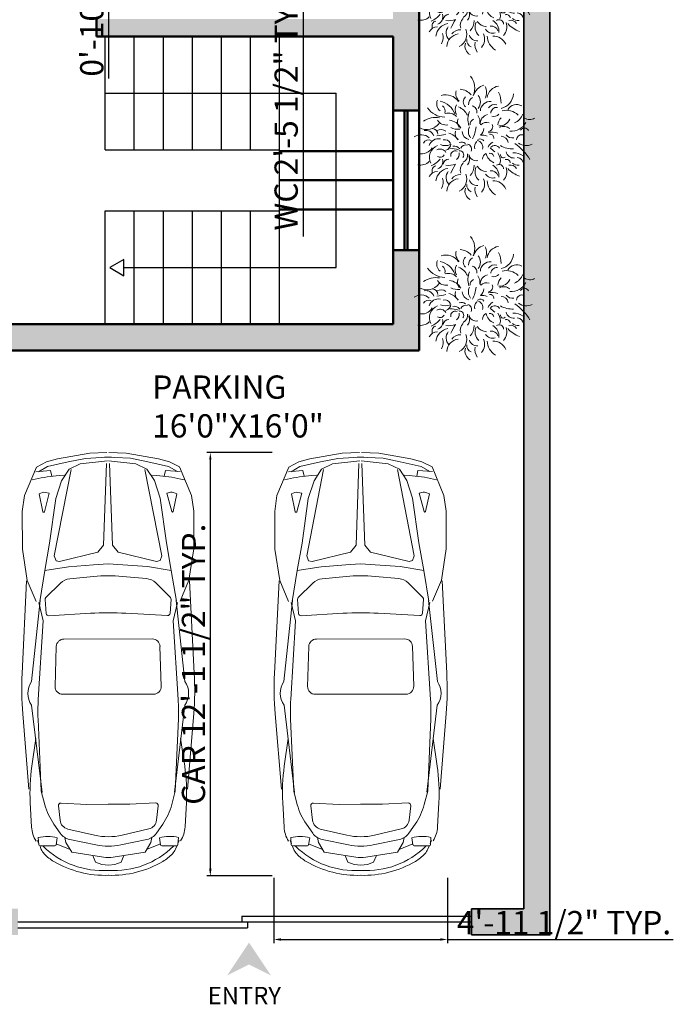
# Model space of a CAD drawing. Units: inches. Extents: x 2442 to 3851, y 589 to 2836.
# Tile 6 of 22: x 2911 to 3136, y 1378 to 1717. Entities that reach past the tile are written whole.
import ezdxf

# ---------------------------------------------------------------- set-up
doc = ezdxf.new("R2010")
doc.units = ezdxf.units.IN
for name, color, linetype, lineweight in [('A-ANNO-DIMS', 2, 'Continuous', 18), ('A-ANNO-SYMB', 1, 'Continuous', 18), ('A-ANNO-TEXT', 7, 'Continuous', 18), ('A-AREA-IDEN', 7, 'Continuous', 18), ('A-EQPM', 9, 'Continuous', 18), ('A-FLOR-STRS', 3, 'Continuous', 25), ('A-GLAZ', 1, 'Continuous', 25), ('A-WALL', 7, 'Continuous', 50), ('A-WALL-PATT', 8, 'Continuous', 13), ('C-PROP', 7, 'Continuous', 35), ('L-PLNT', 94, 'Continuous', 18)]:
    doc.layers.add(name, color=color, linetype=linetype, lineweight=lineweight)
doc.styles.add('ATT', font='romans.shx')
doc.styles.get("Standard").update_dxf_attribs({"font": 'arial.ttf'})
doc.dimstyles.new('ISO-25', dxfattribs={"dimtxt": 8, "dimasz": 2.5, "dimexe": 1.25, "dimexo": 0.625, "dimtad": 1, "dimlunit": 3, "dimtxsty": 'Standard', "dimcen": 2.5, "dimadec": 0, "dimazin": 0, "dimtfac": 1, "dimtmove": 0, "dimatfit": 3, "dimfxl": 1, "dimarcsym": 0})

# ---------------------------------------------------------------- blocks, each defined once
blk = doc.blocks.new('A$C4A3239E3')
for p, q in [((1.2507, 1.6335), (2.1522, 1.6799)), ((2.5445, 1.6742), (3.2816, 1.6148)), ((0.1752, 1.399), (0.1867, 1.5408)), ((0.2661, 1.5794), (0.2592, 1.5495)), ((1.4425, 1.5023), (2.2313, 1.5881)), ((2.4629, 1.587), (3.3117, 1.4863)), ((2.7875, 1.5463), (3.0567, 1.5859)), ((3.4104, 1.6024), (3.6491, 1.5899)), ((0.1359, 1.4288), (0.1867, 1.515)), ((0.3963, 1.4117), (0.388, 1.4492)), ((0.3898, 1.477), (0.4021, 1.5106)), ((0.5758, 1.4596), (0.3963, 1.4117)), ((0.4021, 1.5106), (0.5754, 1.4741)), ((1.4497, 1.5063), (1.149, 1.4553)), ((1.2717, 1.3033), (1.4134, 1.4465)), ((1.4329, 1.4538), (1.567, 1.4437)), ((1.4612, 1.5146), (1.6407, 1.4739)), ((1.6407, 1.4739), (2.4076, 1.5225)), ((2.597, 1.5244), (3.3012, 1.4943)), ((3.3012, 1.4943), (3.4322, 1.4598)), ((3.8218, 1.5205), (3.7519, 1.525)), ((3.7813, 1.5317), (3.8128, 1.5185)), ((3.8334, 1.3629), (3.8334, 1.5081)), ((3.8376, 1.5081), (3.8668, 1.4958)), ((0.0905, 1.2265), (0.1359, 1.4288)), ((0.2308, 1.3867), (0.1752, 1.399)), ((1.59, 1.4175), (1.5668, 1.0125)), ((1.8899, 1.3452), (2.2788, 1.3576)), ((3.6217, 1.372), (3.7108, 1.3099)), ((3.7558, 1.3393), (3.8231, 1.3506)), ((3.8137, 1.3503), (3.8686, 1.2144)), ((0.224, 1.314), (0.2207, 1.2655)), ((1.8186, 0.4085), (1.8178, 1.2708)), ((2.3557, 1.283), (2.3566, 0.3973)), ((3.4158, 1.3024), (3.4294, 1.0516)), ((3.4434, 1.3284), (3.584, 1.3121)), ((3.7535, 1.2644), (3.8014, 1.2553)), ((3.8014, 1.2553), (3.8941, 1.199)), ((0.0565, 1.0588), (0.0905, 1.2265)), ((1.2074, 0.9801), (1.2293, 1.2125)), ((3.6693, 1.236), (3.7299, 0.9762)), ((3.7713, 1.2181), (3.8245, 0.9626)), ((3.8941, 1.199), (3.9452, 0.89)), ((0.0481, 0.9038), (0.0565, 1.0588)), ((3.4294, 1.0516), (3.4292, 0.8428)), ((3.9292, 0.9941), (3.9933, 0.9668)), ((3.9933, 0.9668), (4.0172, 0.906)), ((4.0172, 0.906), (4.0211, 0.842)), ((0.0482, 0.7723), (0.0569, 0.6172)), ((3.4299, 0.6309), (3.4292, 0.8396)), ((3.8948, 0.4844), (3.9453, 0.7934)), ((3.9936, 0.7167), (4.0174, 0.7775)), ((4.0174, 0.7775), (4.0211, 0.8416)), ((1.2077, 0.6979), (1.23, 0.4656)), ((3.6701, 0.4469), (3.7301, 0.7068)), ((3.772, 0.465), (3.8248, 0.7206)), ((3.9295, 0.6893), (3.9936, 0.7167)), ((0.0569, 0.6172), (0.0912, 0.4496)), ((1.5911, 0.2613), (1.5671, 0.6662)), ((3.4167, 0.38), (3.4299, 0.6309)), ((3.8022, 0.4279), (3.8948, 0.4844)), ((0.0912, 0.4496), (0.1371, 0.2474)), ((0.2249, 0.3624), (0.2215, 0.4109)), ((3.7543, 0.4187), (3.8022, 0.4279)), ((3.8147, 0.3328), (3.8693, 0.4688)), ((0.2318, 0.2897), (0.1763, 0.2773)), ((1.2726, 0.3749), (1.4146, 0.232)), ((1.8909, 0.3342), (2.2798, 0.3226)), ((3.4444, 0.354), (3.585, 0.3707)), ((3.6228, 0.3107), (3.7117, 0.3731)), ((3.7568, 0.3438), (3.8241, 0.3326)), ((3.8345, 0.3203), (3.8347, 0.1751)), ((0.1371, 0.2474), (0.188, 0.1613)), ((0.1763, 0.2773), (0.1881, 0.1355)), ((0.3975, 0.2651), (0.3892, 0.2275)), ((0.3911, 0.1998), (0.4034, 0.1661)), ((0.5771, 0.2174), (0.3975, 0.2651)), ((0.4034, 0.1661), (0.5767, 0.203)), ((1.451, 0.1722), (1.1502, 0.2226)), ((1.4341, 0.2247), (1.5682, 0.235)), ((1.4625, 0.1639), (1.6419, 0.205)), ((1.6419, 0.205), (2.4089, 0.1579)), ((2.4644, 0.0936), (3.313, 0.1959)), ((3.3024, 0.1879), (3.4334, 0.2226)), ((0.2676, 0.0971), (0.2606, 0.127)), ((1.4438, 0.1762), (2.2328, 0.0919)), ((2.5984, 0.1564), (3.3024, 0.1879)), ((2.7889, 0.1349), (3.0581, 0.0958)), ((3.8231, 0.1627), (3.7532, 0.1581)), ((3.7826, 0.1514), (3.8141, 0.1647)), ((3.8389, 0.1752), (3.8681, 0.1875)), ((1.2522, 0.0446), (2.1538, 0)), ((2.5461, 0.0065), (3.2831, 0.0673)), ((3.4119, 0.0799), (3.6506, 0.0929))]:
    blk.add_line(p, q)
for points in [[(0, 0.8478), (0.0053, 1.0159), (0.0622, 1.3298), (0.0905, 1.4375), (0.1412, 1.5365), (0.4188, 1.6529), (0.572, 1.6743), (0.9399, 1.6743), (1.2458, 1.627), (1.4497, 1.5408)], [(0.0815, 0.8439), (0.1088, 1.11), (0.1609, 1.2182), (0.2737, 1.2906), (0.4463, 1.3472), (0.8811, 1.4091), (1.149, 1.4553), (1.1121, 1.224), (1.0933, 0.9813), (1.085, 0.8389)], [(0.1644, 1.198), (1.0072, 1.3636), (1.0537, 1.3462), (1.0619, 1.3117), (0.9706, 0.937), (0.9035, 0.8818), (0.106, 0.853)], [(0, 0.8281), (0.0056, 0.6601), (0.0632, 0.3462), (0.0916, 0.2386), (0.1426, 0.1398), (0.4204, 0.0239), (0.5737, 0.0028), (0.9415, 0.0032), (1.2473, 0.0511), (1.4511, 0.1377)], [(0.0815, 0.8322), (0.1094, 0.5662), (0.1616, 0.4581), (0.2746, 0.3859), (0.4473, 0.3296), (0.8822, 0.2683), (1.1502, 0.2226), (1.1128, 0.4539), (1.0936, 0.6965), (1.085, 0.8389)], [(0.1651, 0.4782), (1.0082, 0.314), (1.0547, 0.3316), (1.0628, 0.366), (0.9708, 0.7406), (0.9036, 0.7957), (0.1061, 0.8232)]]:
    blk.add_lwpolyline(points)
for centre, radius, start, end in [((2.3053, -1.296), 2.9798, 85.39524, 92.94517), ((1.7104, 1.2122), 1.4899, 166.91658, 176.08111), ((2.3463, 1.4226), 0.2016, 54.64918, 124.77695), ((3.3168, -0.183), 1.7879, 86.99981, 98.3676), ((3.6355, 1.3122), 0.278, 57.32995, 87.18237), ((0.4365, 1.46), 0.0497, 159.97873, 192.53841), ((0.5739, 1.4668), 0.00745, 284.96001, 78.11246), ((1.431, 1.429), 0.0248, 85.71507, 135.30465), ((1.5652, 1.4189), 0.0248, 356.72561, 85.71507), ((2.5206, -0.2618), 1.7879, 87.54913, 93.62371), ((3.2805, 0.8834), 0.596, 55.07004, 75.25506), ((4.0973, 1.4394), 0.3558, 166.09608, 196.35351), ((3.821, 1.5081), 0.0124, 0, 86.33043), ((3.2466, 0.8963), 0.8285, 356.24509, 44.51945), ((3.8091, 1.3584), 0.149, 46.38363, 67.20138), ((3.6181, 1.158), 0.4258, 30.45768, 46.38363), ((1.8923, 1.2708), 0.0745, 91.82012, 179.9989), ((2.2812, 1.2831), 0.0745, 359.92446, 91.82012), ((3.821, 1.3629), 0.0124, 279.60772, 0), ((3.1325, 0.8724), 0.9892, 358.06945, 30.45768), ((1.3776, 1.1985), 0.149, 135.30465, 174.62136), ((3.4406, 1.3037), 0.0248, 83.37601, 183.11504), ((3.5726, 1.2134), 0.0993, 13.12265, 83.37601), ((3.6254, 1.1877), 0.149, 11.76937, 55.07004), ((2.6908, 0.8405), 1.4899, 174.62136, 185.49162), ((4.5417, 0.8423), 2.9798, 176.72561, 183.38736), ((3.1495, 0.8409), 0.596, 346.99033, 13.12265), ((3.2411, 0.841), 0.596, 348.3436, 11.76937), ((1.2382, 0.8392), 1.1919, 176.89416, 183.21881), ((3.6512, 0.8414), 0.298, 350.72464, 9.38834), ((3.2467, 0.7858), 0.8285, 315.59352, 3.86789), ((3.1326, 0.8094), 0.9892, 329.65529, 2.04353), ((1.3783, 0.4799), 0.149, 185.49162, 224.80833), ((1.8931, 0.4086), 0.0745, 180.11408, 268.29286), ((2.2821, 0.397), 0.0745, 268.29286, 0.18852), ((3.5733, 0.4693), 0.0993, 276.73697, 346.99033), ((3.6261, 0.4951), 0.149, 305.04293, 348.3436), ((1.7111, 0.4671), 1.4899, 184.03187, 193.1964), ((3.4415, 0.3787), 0.0248, 176.99794, 276.73697), ((3.2806, 0.7987), 0.596, 284.85791, 305.04293), ((4.0985, 0.2443), 0.3558, 163.75946, 194.01689), ((3.822, 0.3203), 0.0124, 0.11298, 80.50526), ((3.6188, 0.5248), 0.4258, 313.72935, 329.65529), ((0.4377, 0.2169), 0.0497, 167.57457, 200.13424), ((0.5752, 0.2102), 0.00745, 282.00051, 75.15297), ((1.4322, 0.2495), 0.0248, 224.80833, 274.3979), ((1.5663, 0.2598), 0.0248, 274.3979, 3.38736), ((3.8101, 0.3247), 0.149, 292.9116, 313.72935), ((2.5184, 1.9425), 1.7879, 266.48926, 272.56385), ((3.6364, 0.3706), 0.278, 272.9306, 302.78303), ((3.8223, 0.1751), 0.0124, 273.78255, 0.11298), ((2.3011, 2.9762), 2.9798, 267.1678, 274.71773), ((2.3474, 0.2577), 0.2016, 235.33603, 305.46379), ((3.3148, 1.8652), 1.7879, 261.74537, 273.11317)]:
    blk.add_arc(centre, radius, start, end)
blk = doc.blocks.new('12PPLT14')
at = {"color": 0, "linetype": 'ByBlock'}
for centre, radius, start, end in [((-0.1625, 0.4338), 0.1552, 335.42338, 39.95274), ((-0.1402, 0.294), 0.1288, 38.23315, 86.42537), ((0.1087, 0.3325), 0.1308, 106.37374, 163.6865), ((-0.0015, 0.3959), 0.0956, 329.29525, 30.70475), ((0.216, 0.3316), 0.1193, 99.66859, 170.39165), ((-0.2571, 0.2399), 0.1351, 34.26616, 106.81595), ((-0.0808, 0.3868), 0.0897, 165.56758, 227.79776), ((-0.0467, 0.3138), 0.0589, 134.27921, 225.72079), ((0.0083, 0.2908), 0.0696, 119.33325, 181.22886), ((-0.0514, 0.3138), 0.0928, 323.30293, 36.69707), ((0.0506, 0.3121), 0.1678, 356.78729, 29.97058), ((0.1909, 0.3893), 0.1338, 281.73118, 357.12575), ((-0.2631, 0.3606), 0.1778, 213.40239, 269.32603), ((-0.2523, 0.2979), 0.0813, 157.25274, 229.50512), ((-0.3428, 0.1468), 0.1777, 20.65225, 77.76096), ((-0.3207, 0.2361), 0.0583, 342.26722, 49.59176), ((-0.1032, 0.2472), 0.0733, 144.90044, 215.09956), ((-0.223, 0.1138), 0.1758, 29.57176, 63.83952), ((-0.0403, 0.2301), 0.0513, 346.72425, 78.69141), ((0.1238, 0.2336), 0.083, 82.99618, 178.26594), ((0.1649, 0.2288), 0.0631, 73.67704, 147.47467), ((0.1827, 0.2139), 0.0534, 85.26504, 175.26709), ((0.3529, 0.1986), 0.0923, 62.48991, 146.60828), ((-0.3406, -0.0039), 0.1849, 80.33595, 125.13865), ((-0.2335, 0.1217), 0.0961, 42.98149, 106.47768), ((-0.071, 0.1405), 0.0841, 159.83302, 213.57269), ((0.103, 0.1659), 0.1687, 157.06159, 198.70067), ((-0.0525, 0.1406), 0.0902, 350.08193, 37.96222), ((0.1187, 0.1278), 0.0788, 101.63592, 188.43663), ((0.1561, 0.2471), 0.0582, 252.24344, 319.67919), ((0.2797, 0.1152), 0.0882, 134.29745, 179.34897), ((0.2662, 0.1039), 0.1379, 44.52266, 106.50759), ((0.2843, 0.2512), 0.1271, 292.72328, 340.80825), ((0.4652, 0.2401), 0.0779, 232.4069, 301.86228), ((-0.4178, 0.2048), 0.1282, 239.72439, 324.07722), ((-0.3739, 0.0341), 0.0511, 2.46695, 87.47281), ((-0.2521, 0.2046), 0.0894, 212.77707, 278.72234), ((-0.2353, 0.0367), 0.1199, 26.17758, 85.19259), ((-0.1543, 0.2003), 0.1209, 241.52868, 278.43473), ((0.0228, 0.0586), 0.0851, 152.04195, 218.82735), ((0.002, 0.1188), 0.05, 112.17477, 182.9374), ((-0.34, 0.1477), 0.3488, 334.29004, 351.88848), ((-0.0111, 0.0925), 0.0832, 308.53514, 354.91362), ((0.094, 0.072), 0.0659, 70.33255, 137.7683), ((0.1017, 0.1024), 0.045, 282.88154, 24.03653), ((0.2042, 0.2053), 0.098, 267.79413, 335.77876), ((0.2424, 0.0217), 0.0815, 51.13973, 117.42715), ((0.3092, 0.1973), 0.1353, 263.34537, 334.18502), ((0.4187, 0.0518), 0.0378, 24.37863, 147.98522), ((-0.468, -0.0701), 0.1027, 47.20219, 124.89917), ((-0.4247, -0.0009), 0.0706, 19.83292, 104.60033), ((-0.2974, 0.0074), 0.0691, 53.51258, 119.74743), ((-0.3432, 0.3083), 0.2855, 272.31468, 287.72191), ((-0.2616, -0.0829), 0.132, 32.23561, 76.03189), ((-0.1183, 0.0408), 0.0581, 157.56093, 237.11283), ((-0.0447, 0.0607), 0.0698, 181.7454, 260.02375), ((0.0563, -0.0634), 0.0921, 62.79175, 99.69781), ((0.1427, -0.0803), 0.1346, 68.72592, 105.24218), ((0.125, 0.0053), 0.0314, 351.8398, 98.09997), ((0.2201, -0.0419), 0.0605, 6.85101, 91.88687), ((0.3159, 0.0688), 0.0649, 214.68942, 281.6662), ((0.3966, -0.0128), 0.0455, 62.41504, 179.56563), ((-0.465, -0.0212), 0.1099, 256.13919, 328.23561), ((-0.4019, -0.0635), 0.0512, 65.26306, 151.643), ((-0.3178, -0.086), 0.0842, 78.28592, 162.92531), ((-0.2877, -0.1629), 0.109, 111.2663, 206.92487), ((-0.2585, 0.0428), 0.1041, 246.13691, 293.86309), ((-0.2636, -0.0603), 0.0501, 19.5336, 107.28809), ((-0.2726, -0.0426), 0.0609, 285.53975, 354.90835), ((-0.1835, -0.1238), 0.059, 37.38554, 100.49906), ((-0.1211, -0.079), 0.0486, 46.81003, 114.24578), ((-0.0834, -0.1038), 0.0488, 74.16701, 155.42913), ((-0.0828, -0.0921), 0.0473, 337.57062, 68.78296), ((0.0687, -0.0762), 0.0776, 139.4669, 188.67411), ((0.0015, -0.0752), 0.0596, 343.19149, 77.68697), ((0.0376, -0.0452), 0.0417, 34.85722, 117.04193), ((0.197, -0.1152), 0.0984, 120.3942, 155.69127), ((0.3403, 0.1226), 0.295, 223.14163, 233.53147), ((0.1639, -0.1068), 0.0471, 29.65158, 136.91476), ((0.3131, 0.1083), 0.1966, 239.63817, 273.34301), ((0.055, -0.4368), 0.4844, 31.85079, 54.27081), ((0.4332, 0.0428), 0.1041, 231.87335, 299.32002), ((-0.3051, -0.1456), 0.0555, 28.56403, 118.62426), ((-0.3049, -0.1199), 0.0412, 237.18619, 328.82945), ((-0.2031, -0.2618), 0.1748, 70.7416, 95.82474), ((-0.1751, -0.1446), 0.0382, 64.59889, 195.07151), ((-0.1983, -0.1346), 0.0584, 307.00435, 10.96098), ((-0.1379, -0.1412), 0.0356, 321.49603, 95.05521), ((-0.1367, -0.1434), 0.0675, 297.46031, 9.45776), ((-0.1261, -0.1768), 0.0743, 318.94457, 21.06007), ((0.0056, -0.1284), 0.0629, 187.60372, 281.90432), ((0.1122, -0.1766), 0.0537, 114.99115, 180.12102), ((0.2021, -0.1018), 0.1155, 193.03502, 246.51688), ((0.1228, -0.1611), 0.0339, 11.25201, 101.31224), ((0.0954, -0.19), 0.1169, 346.83309, 34.71337), ((0.2371, -0.1417), 0.0239, 167.98869, 313.85095), ((0.3301, -0.0984), 0.0696, 193.47929, 272.72308), ((0.3295, -0.2531), 0.1299, 52.41158, 94.15676), ((0.3525, -0.2241), 0.0608, 358.61437, 87.08337), ((-0.4721, -0.1203), 0.1079, 257.32785, 313.21298), ((-0.4582, -0.0549), 0.1957, 293.39465, 321.47421), ((-0.3303, -0.2772), 0.044, 103.55337, 199.89539), ((-0.3545, -0.1945), 0.0737, 295.41723, 13.93701), ((-0.2272, -0.2284), 0.0518, 92.73502, 171.87233), ((-0.2342, -0.0362), 0.1951, 263.47371, 288.55685), ((0.4875, -0.6182), 0.7699, 148.94965, 155.30561), ((-0.0491, -0.2722), 0.0823, 133.29294, 197.24957), ((-0.1342, -0.2328), 0.1218, 315.10673, 1.33197), ((0.0958, -0.2858), 0.1, 154.88084, 226.86789), ((0.0984, -0.1813), 0.1021, 214.34273, 267.49691), ((0.0948, -0.3222), 0.106, 354.64066, 60.41558), ((0.2004, -0.2632), 0.04, 3.12979, 123.69191), ((0.1534, -0.2836), 0.1149, 319.19076, 18.21253), ((0.265, -0.2125), 0.0333, 8.08539, 109.93393), ((0.3002, -0.2876), 0.0597, 31.279, 105.07663), ((0.3711, -0.1347), 0.0953, 234.42972, 271.33095), ((-0.3258, -0.3645), 0.0813, 91.05277, 153.01216), ((-0.2197, -0.3768), 0.1216, 98.93269, 173.56524), ((-0.1666, -0.3361), 0.0858, 141.93744, 222.63897), ((-0.1356, -0.3909), 0.0814, 84.45259, 145.99608), ((-0.1912, -0.3476), 0.1157, 295.67023, 21.36797), ((0.1487, -0.2627), 0.0766, 213.89316, 285.61802), ((0.137, -0.3342), 0.0567, 15.84038, 102.17895), ((0.4504, -0.1006), 0.2342, 221.78679, 251.93539), ((-0.4022, -0.3739), 0.1237, 333.15568, 15.43505), ((-0.1321, -0.4596), 0.1156, 98.85859, 176.18052), ((-0.0165, -0.4023), 0.0586, 172.0702, 247.36769), ((0.0095, -0.3403), 0.0634, 192.71209, 278.21462), ((0.1108, -0.4364), 0.1161, 170.09587, 213.65717), ((-0.0287, -0.3897), 0.1058, 317.77354, 24.75223), ((0.2528, -0.3527), 0.1547, 183.87438, 237.37414), ((0.1506, -0.4799), 0.1168, 23.04059, 91.66621), ((-0.0081, -0.4497), 0.0833, 162.96803, 241.48781)]:
    blk.add_arc(centre, radius, start, end, dxfattribs=at)
at = {"color": 0, "linetype": 'ByBlock', "style": 'ATT'}
for tag, p, flags in [('ITEM', (-1.4111, -3.0457), 3), ('ROOM_NUMBER', (-1.4111, -4.379), 1)]:
    blk.add_attdef(tag, p, '', height=1, dxfattribs=dict(at, flags=flags))
blk = doc.blocks.new('*D156')
at = {"layer": 'A-ANNO-DIMS', "color": 0, "lineweight": -2, "transparency": 16777216}
for p, q in [((3012.46, 1764.86), (3007.39, 1764.86)), ((3008.64, 1762.36), (3008.64, 1737.76)), ((3012.46, 1735.26), (3007.39, 1735.26)), ((3008.64, 1735.26), (3008.64, 1642.05))]:
    blk.add_line(p, q, dxfattribs=at)
at = {"layer": 'A-ANNO-DIMS', "color": 0, "transparency": 16777216}
for points in [[(3008.22, 1762.36), (3009.06, 1762.36), (3008.64, 1764.86)], [(3008.22, 1737.76), (3009.06, 1737.76), (3008.64, 1735.26)]]:
    blk.add_solid(points, dxfattribs=at)
at = {"layer": 'Defpoints', "color": 0, "transparency": 16777216}
for p in [(3013.08, 1764.86), (3008.64, 1735.26), (3013.08, 1735.26)]:
    blk.add_point(p, dxfattribs=at)
at = {"layer": 'A-ANNO-DIMS', "color": 0, "transparency": 16777216, "insert": (3003.88, 1687.4), "char_height": 8, "attachment_point": 5, "rotation": 90}
blk.add_mtext('WC 2\'-5 1/2" TYP.', dxfattribs=at)
blk = doc.blocks.new('*D159')
at = {"layer": 'A-ANNO-DIMS', "color": 0, "lineweight": -2, "transparency": 16777216}
for p, q in [((2942.97, 1764.86), (2940.48, 1764.86)), ((2941.73, 1762.36), (2941.73, 1757.57)), ((2942.97, 1755.07), (2940.48, 1755.07)), ((2941.73, 1755.07), (2941.73, 1696.34))]:
    blk.add_line(p, q, dxfattribs=at)
at = {"layer": 'A-ANNO-DIMS', "color": 0, "transparency": 16777216}
for points in [[(2941.31, 1762.36), (2942.15, 1762.36), (2941.73, 1764.86)], [(2941.31, 1757.57), (2942.15, 1757.57), (2941.73, 1755.07)]]:
    blk.add_solid(points, dxfattribs=at)
at = {"layer": 'Defpoints', "color": 0, "transparency": 16777216}
for p in [(2943.6, 1764.86), (2941.73, 1755.07), (2943.6, 1755.07)]:
    blk.add_point(p, dxfattribs=at)
at = {"layer": 'A-ANNO-DIMS', "color": 0, "transparency": 16777216, "insert": (2937.02, 1724.46), "char_height": 8, "attachment_point": 5, "rotation": 90}
blk.add_mtext('0\'-10" TYP.', dxfattribs=at)
blk = doc.blocks.new('*D168')
at = {"layer": 'A-ANNO-DIMS', "color": 0, "lineweight": -2, "transparency": 16777216}
for p, q in [((2997.98, 1567.76), (2975.51, 1567.76)), ((2976.76, 1565.26), (2976.76, 1424.65)), ((2997.98, 1422.15), (2975.51, 1422.15))]:
    blk.add_line(p, q, dxfattribs=at)
at = {"layer": 'A-ANNO-DIMS', "color": 0, "transparency": 16777216}
for points in [[(2976.35, 1565.26), (2977.18, 1565.26), (2976.76, 1567.76)], [(2976.35, 1424.65), (2977.18, 1424.65), (2976.76, 1422.15)]]:
    blk.add_solid(points, dxfattribs=at)
at = {"layer": 'Defpoints', "color": 0, "transparency": 16777216}
for p in [(2998.6, 1567.76), (2976.76, 1422.15), (2998.6, 1422.15)]:
    blk.add_point(p, dxfattribs=at)
at = {"layer": 'A-ANNO-DIMS', "color": 0, "transparency": 16777216, "insert": (2972, 1494.96), "char_height": 8, "attachment_point": 5, "rotation": 90}
blk.add_mtext('CAR 12\'-1 1/2" TYP.', dxfattribs=at)
blk = doc.blocks.new('*D169')
at = {"layer": 'A-ANNO-DIMS', "color": 0, "lineweight": -2, "transparency": 16777216}
for p, q in [((2998.6, 1421.53), (2998.6, 1399.06)), ((3058.33, 1421.53), (3058.33, 1399.06)), ((3001.1, 1400.31), (3055.83, 1400.31)), ((3058.33, 1400.31), (3136.02, 1400.31))]:
    blk.add_line(p, q, dxfattribs=at)
at = {"layer": 'A-ANNO-DIMS', "color": 0, "transparency": 16777216}
for points in [[(3001.1, 1400.73), (3001.1, 1399.89), (2998.6, 1400.31)], [(3055.83, 1400.73), (3055.83, 1399.89), (3058.33, 1400.31)]]:
    blk.add_solid(points, dxfattribs=at)
at = {"layer": 'Defpoints', "color": 0, "transparency": 16777216}
for p in [(2998.6, 1422.15), (3058.33, 1422.15), (3058.33, 1400.31)]:
    blk.add_point(p, dxfattribs=at)
at = {"layer": 'A-ANNO-DIMS', "color": 0, "transparency": 16777216, "insert": (3098.43, 1405.07), "char_height": 8, "attachment_point": 5}
blk.add_mtext('4\'-11 1/2" TYP.', dxfattribs=at)

msp = doc.modelspace()

# ---------------------------------------------------------------- hatches: boundary and pattern name
at = {"layer": 'A-ANNO-SYMB'}
h = msp.add_hatch(color=256, dxfattribs=at)
h.dxf.hatch_style = 1
h.paths.add_polyline_path([(2990.092, 1391.705), (2997.642, 1387.93), (2990.092, 1399.256), (2982.542, 1387.93)])
at = {"layer": 'A-WALL-PATT'}
h = msp.add_hatch(color=256, dxfattribs=at)
h.dxf.hatch_style = 1
h.paths.add_polyline_path([(2502.599, 1992.864), (2719.571, 1992.864), (2719.687, 1994.649), (2720.167, 1997.319), (2721.479, 1992.864), (2726.325, 1992.864), (2727.448, 1994.93), (2729.005, 1997.153), (2728.372, 1992.864), (2728.871, 1992.864), (2730.114, 1994.505), (2731.833, 1996.09), (2730.966, 1993.206), (2730.864, 1992.864), (2771.772, 1992.864), (2771.887, 1994.649), (2772.368, 1997.319), (2773.68, 1992.864), (2778.526, 1992.864), (2779.649, 1994.93), (2781.206, 1997.153), (2780.572, 1992.864), (2781.072, 1992.864), (2782.315, 1994.505), (2784.034, 1996.09), (2783.167, 1993.206), (2783.065, 1992.864), (2821.282, 1992.864), (2821.398, 1994.649), (2821.878, 1997.319), (2823.19, 1992.864), (2828.036, 1992.864), (2829.159, 1994.93), (2830.716, 1997.153), (2830.083, 1992.864), (2830.582, 1992.864), (2831.825, 1994.505), (2833.544, 1996.09), (2832.677, 1993.206), (2832.575, 1992.864), (2869.287, 1992.864), (2869.403, 1994.649), (2869.884, 1997.319), (2871.195, 1992.864), (2876.042, 1992.864), (2877.165, 1994.93), (2878.721, 1997.153), (2878.088, 1992.864), (2878.587, 1992.864), (2879.83, 1994.505), (2881.55, 1996.09), (2880.682, 1993.206), (2880.58, 1992.864), (2919.335, 1992.864), (2919.451, 1994.649), (2919.932, 1997.319), (2921.243, 1992.864), (2926.09, 1992.864), (2927.213, 1994.93), (2928.77, 1997.153), (2928.136, 1992.864), (2928.635, 1992.864), (2929.878, 1994.505), (2931.598, 1996.09), (2930.73, 1993.206), (2930.628, 1992.864), (2966.155, 1992.864), (2966.27, 1994.649), (2966.751, 1997.319), (2968.063, 1992.864), (2972.909, 1992.864), (2974.032, 1994.93), (2975.589, 1997.153), (2974.955, 1992.864), (2975.455, 1992.864), (2976.698, 1994.505), (2978.417, 1996.09), (2977.55, 1993.206), (2977.448, 1992.864), (3010.53, 1992.864), (3010.646, 1994.649), (3011.127, 1997.319), (3012.438, 1992.864), (3017.285, 1992.864), (3018.408, 1994.93), (3019.964, 1997.153), (3019.331, 1992.864), (3019.83, 1992.864), (3021.073, 1994.505), (3022.793, 1996.09), (3021.925, 1993.206), (3021.823, 1992.864), (3057.996, 1992.864), (3058.45, 1995.382), (3059.191, 1992.864), (3065.64, 1992.864), (3067.287, 1995.216), (3066.94, 1992.864), (3068.717, 1992.864), (3070.116, 1994.153), (3069.728, 1992.864), (3084.599, 1992.864), (3084.599, 1983.791), (3085.291, 1983.828), (3084.599, 1983.434), (3084.599, 1932.114), (3085.291, 1932.151), (3084.599, 1931.757), (3084.599, 1886.278), (3085.291, 1886.315), (3084.599, 1885.921), (3084.599, 1410.864), (3066.599, 1410.864), (3066.599, 1401.864), (3093.599, 1401.864), (3093.599, 2001.864), (2493.599, 2001.864), (2493.599, 1401.864), (2538.599, 1401.864), (2538.599, 1410.864), (2502.599, 1410.864)])
h.paths.add_polyline_path([(2738.599, 1410.864), (2547.599, 1410.864), (2547.599, 1401.864), (2738.599, 1401.864)], flags=17)
h.paths.add_polyline_path([(2910.599, 1410.864), (2792.599, 1410.864), (2792.599, 1401.864), (2910.599, 1401.864), (2910.599, 1402.864)], flags=17)
h = msp.add_hatch(color=256, dxfattribs=at)
h.dxf.hatch_style = 1
h.paths.add_polyline_path([(2799.599, 1467.864), (2775.599, 1467.864), (2775.599, 1458.864), (2799.599, 1458.864)])
h.paths.add_polyline_path([(2703.599, 1506.864), (2670.599, 1506.864), (2670.599, 1497.864), (2694.599, 1497.864), (2694.599, 1458.864), (2733.599, 1458.864), (2733.599, 1467.864), (2709.417, 1467.864), (2703.599, 1467.864)])
h.paths.add_polyline_path([(2604.599, 1506.864), (2593.599, 1506.864), (2593.599, 1497.864), (2604.599, 1497.864)])
h.paths.add_polyline_path([(2547.599, 1497.864), (2553.599, 1497.864), (2553.599, 1506.864), (2547.599, 1506.864), (2547.599, 1530.864), (2538.599, 1530.864), (2538.599, 1401.864), (2547.599, 1401.864)])
h.paths.add_polyline_path([(2547.599, 1683.864), (2538.599, 1683.864), (2538.599, 1578.864), (2547.599, 1578.864), (2547.599, 1602.864), (2694.599, 1602.864), (2694.599, 1554.864), (2703.599, 1554.864), (2703.599, 1716.864), (2694.599, 1716.864), (2694.599, 1611.864), (2547.599, 1611.864)])
h.paths.add_polyline_path([(2892.599, 1497.864), (2883.599, 1497.864), (2883.599, 1488.228), (2883.599, 1467.864), (2865.599, 1467.864), (2865.599, 1458.864), (2892.599, 1458.864)])
h.paths.add_polyline_path([(3048.599, 1722.864), (3039.599, 1722.864), (3039.599, 1716.864), (2937.599, 1716.864), (2937.599, 1710.864), (3039.599, 1710.864), (3039.599, 1685.364), (3048.599, 1685.364)])
h.paths.add_polyline_path([(3048.599, 1779.864), (3039.599, 1779.864), (3039.599, 1773.864), (2961.599, 1773.864), (2961.599, 1791.864), (2955.599, 1791.864), (2955.599, 1773.864), (2895.599, 1773.864), (2895.599, 1821.864), (2916.599, 1821.864), (2916.599, 1827.864), (2889.599, 1827.864), (2889.599, 1773.864), (2886.599, 1773.864), (2886.599, 1764.864), (2937.599, 1764.864), (2937.599, 1746.864), (2943.599, 1746.864), (2943.599, 1764.864), (2956.06, 1764.864), (3039.599, 1764.864), (3039.599, 1758.864), (3048.599, 1758.864)])
h.paths.add_polyline_path([(3048.599, 1827.864), (2976.475, 1827.864, -0.1284593), (2975.705, 1827.665), (2964.694, 1827.687, -0.1198794), (2963.972, 1827.864), (2946.599, 1827.864), (2946.599, 1821.864), (3039.599, 1821.864), (3039.599, 1815.864), (3048.599, 1815.864)])
h.paths.add_polyline_path([(3048.599, 1956.864), (3023.366, 1956.864), (3023.277, 1956.402), (3023.088, 1956.864), (3019.494, 1956.864), (3019.543, 1955.479), (3019.146, 1956.864), (3015.599, 1956.864), (3015.599, 1947.864), (3039.599, 1947.864), (3039.599, 1875.864), (3048.599, 1875.864), (3048.599, 1880.743), (3047.576, 1881.614), (3046.081, 1883.417), (3044.931, 1885.453), (3047.541, 1883.949), (3048.599, 1883.343), (3048.599, 1910.588), (3047.049, 1909.235), (3047.896, 1910.862), (3048.599, 1911.909), (3048.599, 1918.826), (3042.477, 1917.032), (3043.928, 1918.154), (3045.59, 1919.165), (3047.525, 1920.009), (3048.599, 1920.305), (3048.599, 1926.579), (3047.576, 1927.45), (3046.081, 1929.252), (3044.931, 1931.289), (3047.541, 1929.785), (3048.599, 1929.179)])
h.paths.add_polyline_path([(2967.599, 1956.864), (2932.171, 1956.864), (2932.082, 1956.402), (2931.893, 1956.864), (2928.299, 1956.864), (2928.348, 1955.479), (2927.951, 1956.864), (2898.599, 1956.864), (2898.599, 1947.864), (2967.599, 1947.864)])
h.paths.add_polyline_path([(2850.599, 1956.864), (2834.118, 1956.864), (2834.029, 1956.402), (2833.84, 1956.864), (2830.245, 1956.864), (2830.294, 1955.479), (2829.897, 1956.864), (2796.599, 1956.864), (2796.599, 1947.864), (2799.599, 1947.864), (2838.599, 1947.864), (2838.599, 1827.864), (2835.599, 1827.864), (2835.599, 1824.864), (2835.599, 1818.864), (2838.599, 1818.864), (2838.599, 1764.864), (2850.599, 1764.864), (2850.599, 1770.864), (2850.599, 1773.864), (2847.599, 1773.864), (2847.599, 1947.864), (2850.599, 1947.864)])
h.paths.add_polyline_path([(2700.599, 1947.864), (2730.599, 1947.864), (2730.599, 1956.864), (2700.599, 1956.864), (2700.599, 1992.864), (2691.599, 1992.864), (2691.599, 1932.864), (2670.599, 1932.864), (2670.599, 1923.864), (2691.599, 1923.864), (2691.599, 1818.864), (2799.599, 1818.864), (2799.599, 1827.864), (2700.599, 1827.864)])
h.paths.add_polyline_path([(2640.599, 1932.864), (2538.599, 1932.864), (2538.599, 1868.364), (2547.599, 1868.364), (2547.599, 1923.864), (2640.599, 1923.864), (2640.599, 1929.864)])
h.paths.add_polyline_path([(2547.599, 1820.364), (2538.599, 1820.364), (2538.599, 1731.864), (2547.599, 1731.864), (2547.599, 1755.864), (2694.599, 1755.864), (2694.599, 1752.864), (2697.599, 1752.864), (2703.599, 1752.864), (2703.599, 1764.864), (2547.599, 1764.864)])
h.paths.add_polyline_path([(2725.858, 1838.187), (2790.115, 1838.187), (2790.115, 1868.602), (2725.858, 1868.602)], flags=25)
h.paths.add_polyline_path([(2892.599, 1671.864), (2883.599, 1671.864), (2883.599, 1563.864), (2892.599, 1563.864), (2892.599, 1602.864), (3048.599, 1602.864), (3048.599, 1637.364), (3039.599, 1637.364), (3039.599, 1611.864), (2892.599, 1611.864)])

# ---------------------------------------------------------------- linework, layer by layer
at = {"layer": 'A-FLOR-STRS'}
for p, q in [((2940.599, 1671.864), (2940.599, 1710.864)), ((2950.599, 1671.864), (2950.599, 1710.864)), ((2960.599, 1671.864), (2960.599, 1710.864)), ((2970.599, 1671.864), (2970.599, 1710.864)), ((2980.599, 1671.864), (2980.599, 1710.864)), ((2990.599, 1671.864), (2990.599, 1710.864)), ((3000.599, 1650.864), (3000.599, 1710.864)), ((2940.599, 1691.364), (3020.099, 1691.364)), ((3020.099, 1631.364), (3020.099, 1691.364)), ((2940.599, 1671.864), (3000.599, 1671.864)), ((2940.599, 1650.864), (3000.599, 1650.864)), ((2947.056, 1631.364), (3020.099, 1631.364))]:
    msp.add_line(p, q, dxfattribs=at)
at = {"layer": 'A-FLOR-STRS', "ltscale": 0.5}
for p, q in [((2940.599, 1611.864), (2940.599, 1650.864)), ((2950.599, 1611.864), (2950.599, 1650.864)), ((2960.599, 1611.864), (2960.599, 1650.864)), ((2970.599, 1611.864), (2970.599, 1650.864)), ((2980.599, 1611.864), (2980.599, 1650.864)), ((2990.599, 1611.864), (2990.599, 1650.864)), ((3000.599, 1611.864), (3000.599, 1650.864))]:
    msp.add_line(p, q, dxfattribs=at)
at = {"layer": 'A-FLOR-STRS'}
msp.add_lwpolyline([(2942.213, 1631.364), (2947.056, 1628.568), (2947.056, 1634.16)], close=True, dxfattribs=at)
at = {"layer": 'A-GLAZ'}
for p, q in [((2910.599, 1406.364), (3066.599, 1406.364)), ((2987.599, 1408.364), (2987.599, 1406.364)), ((2987.599, 1408.364), (3066.599, 1408.364)), ((2989.599, 1406.364), (2989.599, 1404.364)), ((2910.599, 1404.364), (2989.599, 1404.364))]:
    msp.add_line(p, q, dxfattribs=at)
at = {"layer": 'A-WALL'}
for p, q in [((3048.599, 1602.864), (3048.599, 1956.864)), ((2937.599, 1710.864), (2937.599, 1716.864)), ((2937.599, 1710.864), (3039.599, 1710.864)), ((3039.599, 1611.864), (3039.599, 1710.864)), ((3039.599, 1685.364), (3048.599, 1685.364)), ((3043.599, 1637.364), (3043.599, 1685.364)), ((3044.599, 1637.364), (3044.599, 1685.364)), ((3000.599, 1671.364), (3039.599, 1671.364)), ((3000.599, 1661.364), (3039.599, 1661.364)), ((3000.599, 1651.364), (3039.599, 1651.364)), ((3039.599, 1637.364), (3048.599, 1637.364)), ((2892.599, 1611.864), (3039.599, 1611.864)), ((2892.599, 1602.864), (3048.599, 1602.864))]:
    msp.add_line(p, q, dxfattribs=at)
at = {"layer": 'C-PROP'}
msp.add_line((3066.599, 1410.864), (3066.599, 1401.864), dxfattribs=at)
for points in [[(3066.599, 1401.864), (3093.599, 1401.864), (3093.599, 2001.864), (2493.599, 2001.864), (2493.599, 1401.864), (2738.599, 1401.864)], [(3066.599, 1410.864), (3084.599, 1410.864), (3084.599, 1992.864), (2502.599, 1992.864), (2502.599, 1410.864), (2538.599, 1410.864)]]:
    msp.add_lwpolyline(points, dxfattribs=at)

# ---------------------------------------------------------------- block references
at = {"layer": 'A-EQPM', "xscale": 35.27598425228, "yscale": 35.27598425228, "zscale": 35.27598425228, "rotation": 270}
for p in [(2911.994, 1567.762), (2998.833, 1567.762)]:
    msp.add_blockref('A$C4A3239E3', p, dxfattribs=at)
at = {"layer": 'L-PLNT', "xscale": 40.07642696295986, "yscale": 40.07642696295986, "zscale": 40.07642696295986}
for p in [(3068.013, 1725.519), (3068.013, 1675.743), (3068.013, 1620.633)]:
    msp.add_blockref('12PPLT14', p, dxfattribs=at)

# ---------------------------------------------------------------- texts
at = {"layer": 'A-ANNO-TEXT', "insert": (2975.874, 1384.023), "char_height": 6, "attachment_point": 1}
msp.add_mtext_dynamic_manual_height_columns('{\\fTimes New Roman|b0|i0|c0|p18;ENTRY}', width=196.26071, gutter_width=12.5, heights=[0], dxfattribs=at)
at = {"layer": 'A-AREA-IDEN', "insert": (2956.774, 1594.257), "char_height": 8, "attachment_point": 1}
msp.add_mtext_dynamic_manual_height_columns('{\\fTimes New Roman|b0|i0|c0|p18;PARKING\\P16\'0"X16\'0"}', width=110.76054, gutter_width=12.5, heights=[0], dxfattribs=at)

# ---------------------------------------------------------------- dimensions: what is measured, and where the dimension line sits
at = {"layer": 'A-ANNO-DIMS'}
for base, p1, p2, text, picture, middle in [((2941.729, 1755.073), (2943.599, 1764.864), (2943.599, 1755.073), '<> TYP.', '*D159', (2937.02, 1724.458)), ((3008.641, 1735.257), (3013.083, 1764.864), (3013.083, 1735.257), 'WC <> TYP.', '*D156', (3003.88, 1687.403)), ((2976.763, 1422.15), (2998.605, 1567.762), (2998.605, 1422.15), 'CAR <> TYP.', '*D168', (2972.002, 1494.956))]:
    dim = msp.add_linear_dim(base=base, p1=p1, p2=p2, angle=270, text=text, dimstyle='ISO-25', override={"dimdec": 1, "dimrnd": 0, "dimzin": 1, "dimlunit": 4, "dimfrac": 2}, dxfattribs=at)
    dim.commit()
    dim.dimension.update_dxf_attribs({"geometry": picture, "text_midpoint": middle})
dim = msp.add_linear_dim(base=(3058.331, 1400.308), p1=(2998.605, 1422.15), p2=(3058.331, 1422.15), text='<> TYP.', dimstyle='ISO-25', override={"dimdec": 1, "dimrnd": 0, "dimzin": 1, "dimlunit": 4, "dimfrac": 2}, dxfattribs=at)
dim.commit()
dim.dimension.update_dxf_attribs({"geometry": '*D169', "text_midpoint": (3098.427, 1405.07)})

doc.saveas('drawing.dxf')
